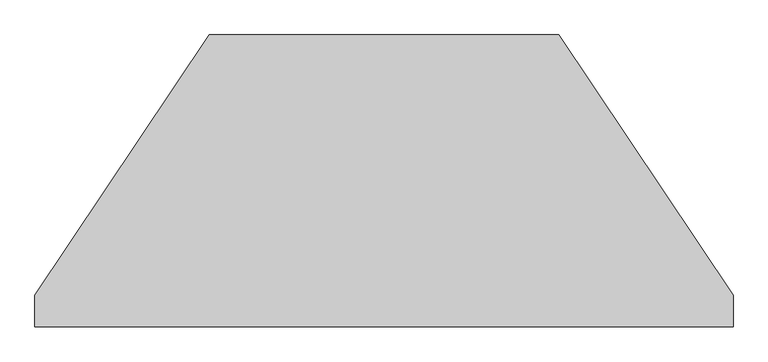
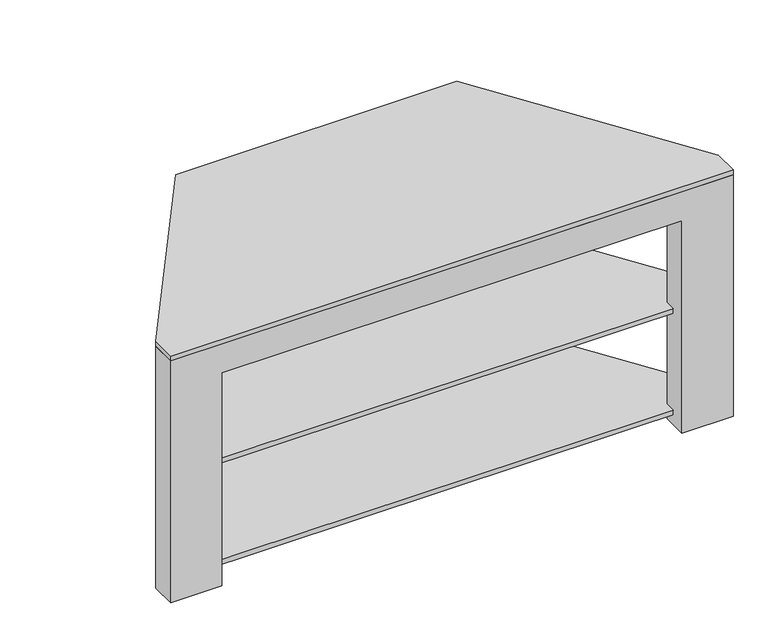
"""IFC4 building model written with IfcOpenShell, lengths in millimetres: furniture geometry."""

from ifc_helpers import new_model, si_unit, point, frame, frame_2d, origin, place, context, project, spatial, polyline, circle_curve, trimmed, segment, composite_curve, outline, extrude, faceted_brep, source, transform, mapped, element, save


def furniture_40ec15d9(model_context):
    return source(origin(), model_context, "Body", "SolidModel", [
        extrude(outline(polyline([(420.3099533, -30.0), (625.1880021, -335.4545455), (625.1880021, -430.0), (-374.8119979, -430.0), (-374.8119979, -335.4545455), (-169.9339492, -30.0), (420.3099533, -30.0)])), frame((0.0, 0.0, 20.0), z_axis=(0.0, 0.0, 1.0), x_axis=(1.0, 0.0, 0.0)), (0.0, 0.0, 1.0), 10.0),
        extrude(outline(polyline([(420.3099533, -30.0), (625.1880021, -335.4545455), (625.1880021, -430.0), (-374.8119979, -430.0), (-374.8119979, -335.4545455), (-169.9339492, -30.0), (420.3099533, -30.0)])), frame((0.0, 0.0, 230.0), z_axis=(0.0, 0.0, 1.0), x_axis=(1.0, 0.0, 0.0)), (0.0, 0.0, 1.0), 10.0),
        extrude(outline(polyline([(400.1880021, 0.0), (675.1880021, -410.0), (675.1880021, -460.0), (-424.8119979, -460.0), (-424.8119979, -410.0), (-149.8119979, 0.0), (400.1880021, 0.0)])), frame((0.0, 0.0, 500.0), z_axis=(0.0, 0.0, 1.0), x_axis=(1.0, 0.0, 0.0)), (0.0, 0.0, 1.0), 10.0),
        extrude(outline(polyline([(-50.0, 500.0), (0.0, 500.0), (0.0, 0.0), (-50.0, 0.0), (-50.0, 20.0), (-30.0, 20.0), (-30.0, 30.0), (-50.0, 30.0), (-50.0, 230.0), (-30.0, 230.0), (-30.0, 240.0), (-50.0, 240.0), (-50.0, 500.0)])), frame((-149.8119979, 0.0, 0.0), z_axis=(1.0, 0.0, 0.0), x_axis=(0.0, 1.0, 0.0)), (0.0, 0.0, 1.0), 100.0),
        extrude(outline(polyline([(-50.0, 500.0), (0.0, 500.0), (0.0, 0.0), (-50.0, 0.0), (-50.0, 20.0), (-30.0, 20.0), (-30.0, 30.0), (-50.0, 30.0), (-50.0, 230.0), (-30.0, 230.0), (-30.0, 240.0), (-50.0, 240.0), (-50.0, 500.0)])), frame((300.1880021, 0.0, 0.0), z_axis=(1.0, 0.0, 0.0), x_axis=(0.0, 1.0, 0.0)), (0.0, 0.0, 1.0), 100.0),
        faceted_brep([(-424.8119979, -460.0, 0.0), (-324.8119979, -460.0, 0.0), (-324.8119979, -460.0, 440.0), (575.1880021, -460.0, 440.0), (575.1880021, -460.0, 0.0), (675.1880021, -460.0, 0.0), (675.1880021, -460.0, 500.0), (-424.8119979, -460.0, 500.0), (-424.8119979, -410.0, 0.0), (-424.8119979, -410.0, 500.0), (675.1880021, -410.0, 500.0), (675.1880021, -410.0, 0.0), (575.1880021, -410.0, 0.0), (575.1880021, -410.0, 20.0), (625.1880021, -410.0, 20.0), (625.1880021, -410.0, 30.0), (575.1880021, -410.0, 30.0), (575.1880021, -410.0, 230.0), (625.1880021, -410.0, 230.0), (625.1880021, -410.0, 240.0), (575.1880021, -410.0, 240.0), (575.1880021, -410.0, 440.0), (-324.8119979, -410.0, 440.0), (-324.8119979, -410.0, 240.0), (-374.8119979, -410.0, 240.0), (-374.8119979, -410.0, 230.0), (-324.8119979, -410.0, 230.0), (-324.8119979, -410.0, 30.0), (-374.8119979, -410.0, 30.0), (-374.8119979, -410.0, 20.0), (-324.8119979, -410.0, 20.0), (-324.8119979, -410.0, 0.0), (-324.8119979, -430.0, 20.0), (-324.8119979, -430.0, 30.0), (-324.8119979, -430.0, 230.0), (-324.8119979, -430.0, 240.0), (575.1880021, -430.0, 240.0), (575.1880021, -430.0, 230.0), (575.1880021, -430.0, 30.0), (575.1880021, -430.0, 20.0), (625.1880021, -430.0, 240.0), (-374.8119979, -430.0, 240.0), (-374.8119979, -430.0, 230.0), (625.1880021, -430.0, 230.0), (625.1880021, -430.0, 30.0), (-374.8119979, -430.0, 30.0), (-374.8119979, -430.0, 20.0), (625.1880021, -430.0, 20.0)], [[[0, 1, 2, 3, 4, 5, 6, 7]], [[8, 9, 10, 11, 12, 13, 14, 15, 16, 17, 18, 19, 20, 21, 22, 23, 24, 25, 26, 27, 28, 29, 30, 31]], [[1, 0, 8, 31]], [[2, 1, 31, 30, 32, 33, 27, 26, 34, 35, 23, 22]], [[3, 2, 22, 21]], [[4, 3, 21, 20, 36, 37, 17, 16, 38, 39, 13, 12]], [[5, 4, 12, 11]], [[6, 5, 11, 10]], [[7, 6, 10, 9]], [[0, 7, 9, 8]], [[19, 40, 36, 20]], [[35, 41, 24, 23]], [[25, 42, 34, 26]], [[37, 43, 18, 17]], [[41, 42, 25, 24]], [[42, 41, 35, 34]], [[40, 43, 37, 36]], [[43, 40, 19, 18]], [[15, 44, 38, 16]], [[33, 45, 28, 27]], [[29, 46, 32, 30]], [[39, 47, 14, 13]], [[45, 46, 29, 28]], [[46, 45, 33, 32]], [[44, 47, 39, 38]], [[47, 44, 15, 14]]]),
        extrude(outline(polyline([(0.0, 300.1880021), (500.0, 300.1880021), (500.0, -49.8119979), (0.0, -49.8119979), (0.0, 300.1880021)]), holes=[composite_curve([segment(polyline([(245.0, 145.1700818), (245.0, 105.2059224)]), True, "CONTINUOUS"), segment(trimmed(circle_curve(frame_2d((257.5, 105.2059224)), 12.5), [point((245.0, 105.2059224))], [point((270.0, 105.2059224))], True, "CARTESIAN"), True, "CONTINUOUS"), segment(polyline([(270.0, 105.2059224), (270.0, 145.1700818)]), True, "CONTINUOUS"), segment(trimmed(circle_curve(frame_2d((257.5, 145.1700818)), 12.5), [point((270.0, 145.1700818))], [point((245.0, 145.1700818))], True, "CARTESIAN"), True, "CONTINUOUS")], self_intersect=False), composite_curve([segment(polyline([(35.0, 145.1880021), (35.0, 105.2059224)]), True, "CONTINUOUS"), segment(trimmed(circle_curve(frame_2d((47.5, 105.2059224)), 12.5), [point((35.0, 105.2059224))], [point((60.0, 105.2059224))], True, "CARTESIAN"), True, "CONTINUOUS"), segment(polyline([(60.0, 105.2059224), (60.0, 145.1880021)]), True, "CONTINUOUS"), segment(trimmed(circle_curve(frame_2d((47.5, 145.1880021)), 12.5), [point((60.0, 145.1880021))], [point((35.0, 145.1880021))], True, "CARTESIAN"), True, "CONTINUOUS")], self_intersect=False)]), frame((0.0, -30.0, 0.0), z_axis=(0.0, 1.0, 0.0), x_axis=(0.0, 0.0, 1.0)), (0.0, 0.0, 1.0), 10.0),
    ])


if __name__ == "__main__":
    model = new_model("IFC4")
    model_context = context("Model", 3, world=origin())
    ifc_project = project(units=[si_unit("LENGTHUNIT", "METRE", prefix="MILLI")], contexts=[model_context])
    site = spatial("IfcSite", under=ifc_project)
    building = spatial("IfcBuilding", under=site)
    placement = place(None, origin())
    furniture_shape = furniture_40ec15d9(model_context)
    element("IfcFurniture", 1, at=placement, inside=building, context=model_context, shape_type="MappedRepresentation", body=[
        mapped(furniture_shape, transform((0.0, 0.0, 0.0), x_axis=(1.0, 0.0, 0.0), y_axis=(0.0, 1.0, 0.0), z_axis=(0.0, 0.0, 1.0))),
    ])
    save(model, "model.ifc")

# Revit data of these elements
# Type
#   Depth = 460 mm
#   Width = 1100 mm
#   Height = 500 mm
#   Finish = Melamine - Gray
#   Default Elevation = 0
# Element 1 (IfcFurniture)
#   Materials on its faces: "Melamine - Gray", "Glass - Shelves"
# Materials
#   "Melamine - Gray": class "Wood", colour RGB 49 49 49, transparency 0
#   "Glass - Shelves": class "Glass", colour RGB 167 167 167, transparency 0.9
